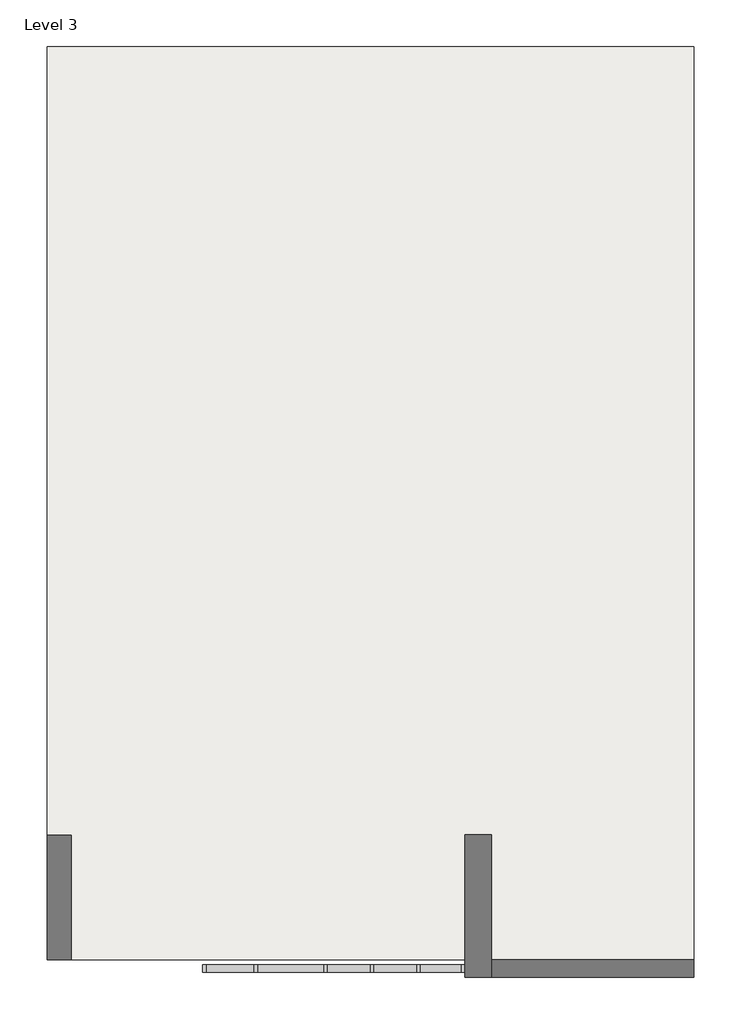
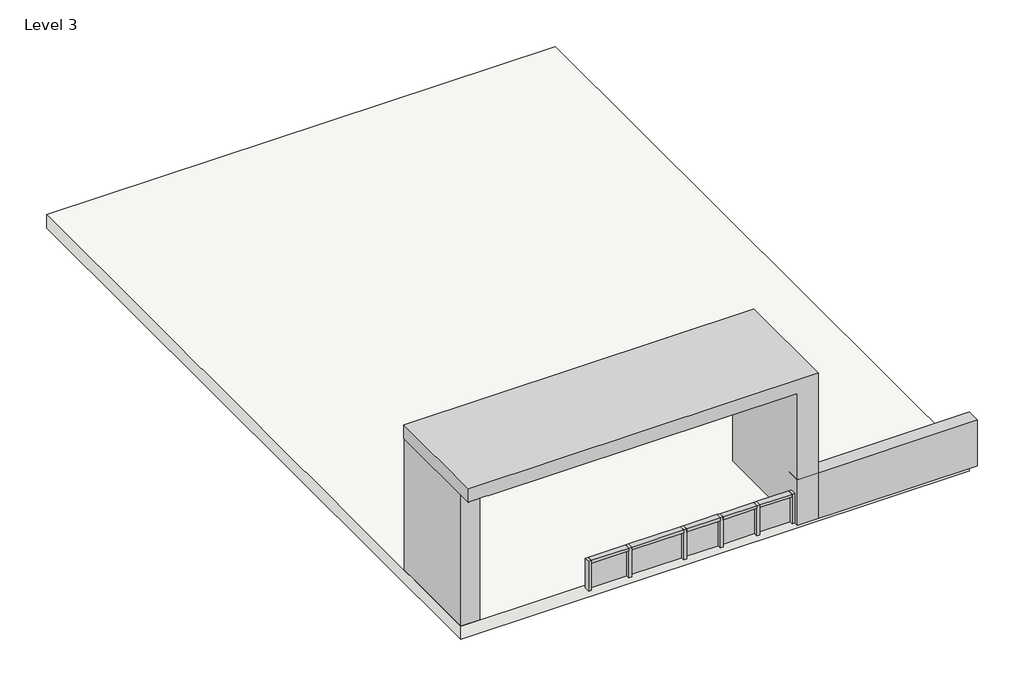
# One storey: 11 members, 5 plates, 3 proxies, 1 roof.
"""IFC4 building model written with IfcOpenShell, lengths in millimetres."""

from ifc_helpers import new_model, si_unit, frame, origin, place, context, project, spatial, polyline, outline, extrude, transform, mapped, element, save
from components import generic_models_4_generic_models_4_e1efe8a4, generic_models_5_generic_models_5_b383e08d, generic_models_6_generic_models_6_a941f71c, member_c17f1be2, member_106f6fb5, member_dae533be, member_11cde41b, member_38fa7f05, member_0d9ba275, system_panel_glazed_c1eeadb6, system_panel_glazed_69f0b79b, system_panel_glazed_f6fef574, system_panel_glazed_daf883b7

model = new_model("IFC4")

# Units and contexts
model_context = context("Model", 3, world=origin())
ifc_project = project(units=[si_unit("LENGTHUNIT", "METRE", prefix="MILLI")], contexts=[model_context])

# Site, building, storey
site = spatial("IfcSite", under=ifc_project)
building = spatial("IfcBuilding", under=site)
storey = spatial("IfcBuildingStorey", under=building, Name="Level 3", Elevation=6096.0)

# Proxies
placement = place(None, origin())
generic_models_4_generic_models_4_shape = generic_models_4_generic_models_4_e1efe8a4(model_context)
element("IfcBuildingElementProxy", 1, Name="Generic Models 4 : Generic Models 4", ObjectType="Generic Models 4 : Generic Models 4", at=placement, inside=storey, context=model_context, shape_type="MappedRepresentation", body=[
    mapped(generic_models_4_generic_models_4_shape, transform((0.0, 0.0, 0.0), x_axis=(1.0, 0.0, 0.0), y_axis=(0.0, 1.0, 0.0), z_axis=(0.0, 0.0, 1.0))),
])
generic_models_5_generic_models_5_shape = generic_models_5_generic_models_5_b383e08d(model_context)
element("IfcBuildingElementProxy", 2, Name="Generic Models 5 : Generic Models 5", ObjectType="Generic Models 5 : Generic Models 5", at=placement, inside=storey, context=model_context, shape_type="MappedRepresentation", body=[
    mapped(generic_models_5_generic_models_5_shape, transform((0.0, 0.0, 0.0), x_axis=(1.0, 0.0, 0.0), y_axis=(0.0, 1.0, 0.0), z_axis=(0.0, 0.0, 1.0))),
])
generic_models_6_generic_models_6_shape = generic_models_6_generic_models_6_a941f71c(model_context)
element("IfcBuildingElementProxy", 3, Name="Generic Models 6 : Generic Models 6", ObjectType="Generic Models 6 : Generic Models 6", at=placement, inside=storey, context=model_context, shape_type="MappedRepresentation", body=[
    mapped(generic_models_6_generic_models_6_shape, transform((0.0, 0.0, 0.0), x_axis=(1.0, 0.0, 0.0), y_axis=(0.0, 1.0, 0.0), z_axis=(0.0, 0.0, 1.0))),
])

# Members
member_shape = member_c17f1be2(model_context)
element("IfcMember", 4, ObjectType="Rectangular Mullion : 2.5\" x 5\" rectangular", at=placement, inside=storey, context=model_context, shape_type="MappedRepresentation", body=[
    mapped(member_shape, transform((-13449.7668407, -15486.1742702, 7091.4281505), x_axis=(0.0, 0.0, 1.0), y_axis=(0.0, -1.0, 0.0), z_axis=(1.0, 0.0, 0.0))),
])
member_2_shape = member_106f6fb5(model_context)
element("IfcMember", 5, ObjectType="Rectangular Mullion : 2.5\" x 5\" rectangular", at=placement, inside=storey, context=model_context, shape_type="MappedRepresentation", body=[
    mapped(member_2_shape, transform((-10617.7434105, -15486.1742702, 6400.8), x_axis=(1.0, 0.0, 0.0), y_axis=(0.0, -1.0, 0.0), z_axis=(0.0, 0.0, -1.0))),
])
element("IfcMember", 6, ObjectType="Rectangular Mullion : 2.5\" x 5\" rectangular", at=placement, inside=storey, context=model_context, shape_type="MappedRepresentation", body=[
    mapped(member_2_shape, transform((-11417.8215334, -15486.1742702, 6400.8), x_axis=(1.0, 0.0, 0.0), y_axis=(0.0, -1.0, 0.0), z_axis=(0.0, 0.0, -1.0))),
])
element("IfcMember", 7, ObjectType="Rectangular Mullion : 2.5\" x 5\" rectangular", at=placement, inside=storey, context=model_context, shape_type="MappedRepresentation", body=[
    mapped(member_2_shape, transform((-12217.8996563, -15486.1742702, 6400.8), x_axis=(1.0, 0.0, 0.0), y_axis=(0.0, -1.0, 0.0), z_axis=(0.0, 0.0, -1.0))),
])
element("IfcMember", 8, ObjectType="Rectangular Mullion : 2.5\" x 5\" rectangular", at=placement, inside=storey, context=model_context, shape_type="MappedRepresentation", body=[
    mapped(member_2_shape, transform((-13418.0168407, -15486.1742702, 6400.8), x_axis=(1.0, 0.0, 0.0), y_axis=(0.0, -1.0, 0.0), z_axis=(0.0, 0.0, -1.0))),
])
member_3_shape = member_dae533be(model_context)
element("IfcMember", 9, ObjectType="Rectangular Mullion : 2.5\" x 5\" rectangular", at=placement, inside=storey, context=model_context, shape_type="MappedRepresentation", body=[
    mapped(member_3_shape, transform((-10649.4934105, -15486.1742702, 7091.4281505), x_axis=(0.0, 0.0, 1.0), y_axis=(0.0, -1.0, 0.0), z_axis=(1.0, 0.0, 0.0))),
])
element("IfcMember", 10, ObjectType="Rectangular Mullion : 2.5\" x 5\" rectangular", at=placement, inside=storey, context=model_context, shape_type="MappedRepresentation", body=[
    mapped(member_3_shape, transform((-11449.5715334, -15486.1742702, 7091.4281505), x_axis=(0.0, 0.0, 1.0), y_axis=(0.0, -1.0, 0.0), z_axis=(1.0, 0.0, 0.0))),
])
member_4_shape = member_11cde41b(model_context)
element("IfcMember", 11, ObjectType="Rectangular Mullion : 2.5\" x 5\" rectangular", at=placement, inside=storey, context=model_context, shape_type="MappedRepresentation", body=[
    mapped(member_4_shape, transform((-12249.6496563, -15486.1742702, 7091.4281505), x_axis=(0.0, 0.0, 1.0), y_axis=(0.0, -1.0, 0.0), z_axis=(1.0, 0.0, 0.0))),
])
member_5_shape = member_38fa7f05(model_context)
element("IfcMember", 12, ObjectType="Rectangular Mullion : 2.5\" x 5\" rectangular", at=placement, inside=storey, context=model_context, shape_type="MappedRepresentation", body=[
    mapped(member_5_shape, transform((-14332.4168407, -15486.1742702, 7091.4281505), x_axis=(-1.0, 0.0, 0.0), y_axis=(0.0, -1.0, 0.0), z_axis=(0.0, 0.0, 1.0))),
])
member_6_shape = member_0d9ba275(model_context)
element("IfcMember", 13, ObjectType="Rectangular Mullion : 2.5\" x 5\" rectangular", at=placement, inside=storey, context=model_context, shape_type="MappedRepresentation", body=[
    mapped(member_6_shape, transform((-9881.1652876, -15486.1742702, 7091.4281505), x_axis=(0.0, 0.0, 1.0), y_axis=(0.0, -1.0, 0.0), z_axis=(1.0, 0.0, 0.0))),
])
element("IfcMember", 14, ObjectType="Rectangular Mullion : 2.5\" x 5\" rectangular", at=placement, inside=storey, context=model_context, shape_type="MappedRepresentation", body=[
    mapped(member_5_shape, transform((-9817.6652876, -15486.1742702, 6400.8), x_axis=(1.0, 0.0, 0.0), y_axis=(0.0, -1.0, 0.0), z_axis=(0.0, 0.0, -1.0))),
])

# Plates
system_panel_glazed_shape = system_panel_glazed_c1eeadb6(model_context)
element("IfcPlate", 15, ObjectType="System Panel : Glazed", at=placement, inside=storey, context=model_context, shape_type="MappedRepresentation", body=[
    mapped(system_panel_glazed_shape, transform((-11817.8605949, -15486.1742702, 6400.8), x_axis=(1.0, 0.0, 0.0), y_axis=(0.0, 1.0, 0.0), z_axis=(0.0, 0.0, 1.0))),
])
element("IfcPlate", 16, ObjectType="System Panel : Glazed", at=placement, inside=storey, context=model_context, shape_type="MappedRepresentation", body=[
    mapped(system_panel_glazed_shape, transform((-11017.782472, -15486.1742702, 6400.8), x_axis=(1.0, 0.0, 0.0), y_axis=(0.0, 1.0, 0.0), z_axis=(0.0, 0.0, 1.0))),
])
system_panel_glazed_2_shape = system_panel_glazed_69f0b79b(model_context)
element("IfcPlate", 17, ObjectType="System Panel : Glazed", at=placement, inside=storey, context=model_context, shape_type="MappedRepresentation", body=[
    mapped(system_panel_glazed_2_shape, transform((-12817.9582485, -15486.1742702, 6400.8), x_axis=(1.0, 0.0, 0.0), y_axis=(0.0, 1.0, 0.0), z_axis=(0.0, 0.0, 1.0))),
])
system_panel_glazed_3_shape = system_panel_glazed_f6fef574(model_context)
element("IfcPlate", 18, ObjectType="System Panel : Glazed", at=placement, inside=storey, context=model_context, shape_type="MappedRepresentation", body=[
    mapped(system_panel_glazed_3_shape, transform((-13859.3418407, -15486.1742702, 6400.8), x_axis=(1.0, 0.0, 0.0), y_axis=(0.0, 1.0, 0.0), z_axis=(0.0, 0.0, 1.0))),
])
system_panel_glazed_4_shape = system_panel_glazed_daf883b7(model_context)
element("IfcPlate", 19, ObjectType="System Panel : Glazed", at=placement, inside=storey, context=model_context, shape_type="MappedRepresentation", body=[
    mapped(system_panel_glazed_4_shape, transform((-10233.5793491, -15486.1742702, 6400.8), x_axis=(1.0, 0.0, 0.0), y_axis=(0.0, 1.0, 0.0), z_axis=(0.0, 0.0, 1.0))),
])

# Roof
element("IfcRoof", 20, ObjectType="Generic - 12\"", at=placement, inside=storey, context=model_context, shape_type="SweptSolid", body=[
    extrude(outline(polyline([(-17001.1767684, 363.4257298), (-5875.9767684, 363.4257298), (-5875.9767684, -15333.7742702), (-17001.1767684, -15333.7742702), (-17001.1767684, 363.4257298)])), frame((0.0, 0.0, 6096.0), z_axis=(0.0, 0.0, 1.0), x_axis=(1.0, 0.0, 0.0)), (0.0, 0.0, 1.0), 304.8),
])

save(model, "model.ifc")

# Revit data of these elements
# Type "Rectangular Mullion : 2.5\" x 5\" rectangular"
#   built-in parameter 1007304 = 0.416667 (stored number, unit not read)
#   built-in parameter 1007301 = 0.104167 (stored number, unit not read)
#   built-in parameter 1007300 = 0.104167 (stored number, unit not read)
# Type "System Panel : Glazed"
#   Construction Type Id = "GSP4R"
#   Analytic Construction = "1/8 in Pilkington single glazing"
#   Visual Light Transmittance = 0.9
#   Solar Heat Gain Coefficient = 0.86
#   Heat Transfer Coefficient (U) = 1.18115 BTU/(h·ft²·°F)
#   Define Thermal Properties by = 1
# Type "Generic - 12\""
#   Assembly Code = "B1020"
#   Layers, outside or top first: 1' - 0" no material (function 1)
# Element 1 (IfcBuildingElementProxy, "Generic Models 4 : Generic Models 4")
#   Phase Created = New Construction
# Element 2 (IfcBuildingElementProxy, "Generic Models 5 : Generic Models 5")
#   Phase Created = New Construction
# Element 3 (IfcBuildingElementProxy, "Generic Models 6 : Generic Models 6")
#   Phase Created = New Construction
# Elements 4, 5, 6, 7, 8, 9, 10, 11, 12, 13, 14 (IfcMember, "Rectangular Mullion : 2.5\" x 5\" rectangular")
#   Phase Created = New Construction
#   Materials on its faces: "Aluminum"
# Elements 15, 16, 17, 18, 19 (IfcPlate, "System Panel : Glazed")
#   Phase Created = New Construction
#   Materials on its faces: "Glass"
# Element 20 (IfcRoof, "Generic - 12\"")
#   built-in parameter 1001705 = 21 (stored number, unit not read)
#   built-in parameter 1001710 = 33615
#   Phase Created = New Construction
#   Materials on its faces: "Default Roof"
# Materials
#   "Aluminum": class "Metal", colour RGB 247 247 247, transparency 0, Description = "Aluminum 6061", Cost = 0
#   "Glass": class "Glass", colour RGB 0 128 192, transparency 0.75, Description = "Soda Lime Glass", Cost = 0
#   "Default Roof": colour RGB 88 101 114, transparency 0, Cost = 0
